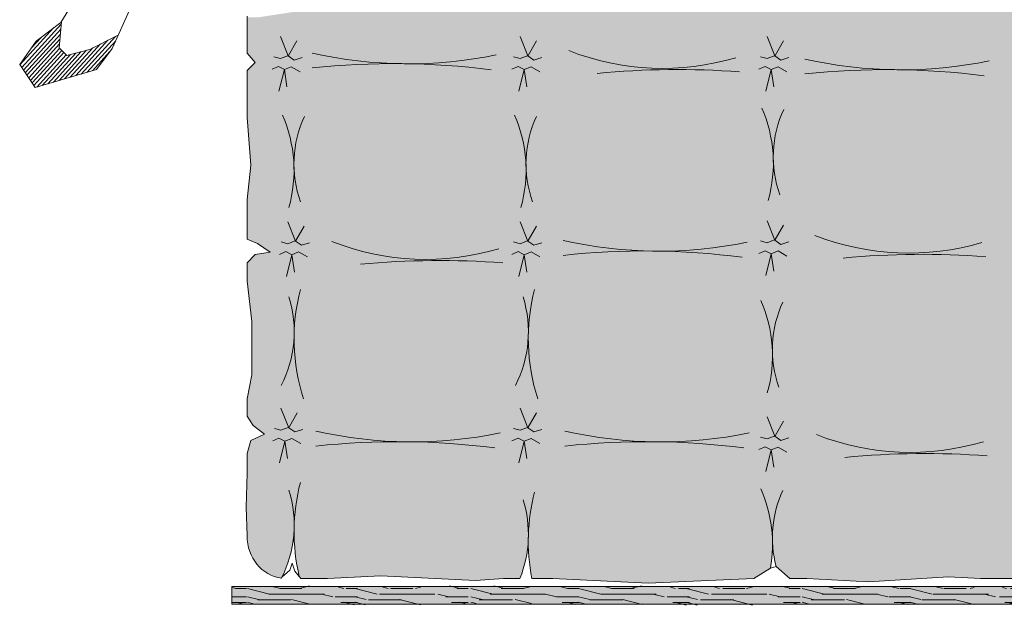
# Model space of a CAD drawing. Units: inches. Extents: x 1994 to 3075, y 3517 to 3950.
# Tile 33 of 58: x 1994.61846 to 1994.66748, y 3553.69193 to 3553.72103. Entities that reach past the tile are written whole.
import ezdxf

# ---------------------------------------------------------------- set-up
doc = ezdxf.new("R2010")
doc.units = ezdxf.units.IN
doc.layers.add('A-FURN-REFR', color=8, linetype='Continuous', lineweight=13)
doc.layers.add('A-FURN-REFR-PATT', color=8, linetype='Continuous', lineweight=13)

msp = doc.modelspace()

# ---------------------------------------------------------------- hatches: boundary and pattern name
at = {"layer": 'A-FURN-REFR-PATT'}
h = msp.add_hatch(color=256, dxfattribs=at)
h.set_gradient(color1=(238, 215, 180), color2=(243, 226, 201), one_color=1, tint=0.87)
edge = h.paths.add_edge_path()
edge.add_line((1994.681542, 3553.709525), (1994.682048, 3553.709217))
edge.add_line((1994.682048, 3553.709217), (1994.682631, 3553.708815))
edge.add_line((1994.682631, 3553.708815), (1994.682631, 3553.708383))
edge.add_line((1994.682631, 3553.708383), (1994.682498, 3553.704652))
edge.add_line((1994.682498, 3553.704652), (1994.682631, 3553.701474))
edge.add_line((1994.682631, 3553.701474), (1994.682631, 3553.700426))
edge.add_line((1994.682631, 3553.700426), (1994.682104, 3553.700396))
edge.add_line((1994.682104, 3553.700396), (1994.681598, 3553.699902))
edge.add_line((1994.681598, 3553.699902), (1994.681992, 3553.699717))
edge.add_line((1994.681992, 3553.699717), (1994.682631, 3553.699439))
edge.add_line((1994.682631, 3553.699439), (1994.682631, 3553.695334))
edge.add_ellipse((1994.680709, 3553.695334), major_axis=(0, 0.002111), ratio=0.910403, start_angle=180, end_angle=270, ccw=False)
edge.add_line((1994.680709, 3553.693223), (1994.680522, 3553.693223))
edge.add_line((1994.680522, 3553.693223), (1994.680314, 3553.694))
edge.add_ellipse((1994.68491, 3553.694998), major_axis=(0, 0.005146), ratio=0.910403, start_angle=92.3431, end_angle=102.2543, ccw=False)
edge.add_ellipse((1994.674568, 3553.694683), major_axis=(0, 0.006219), ratio=0.910403, start_angle=-88.7485, end_angle=-87.76)
edge.add_ellipse((1994.68491, 3553.694998), major_axis=(0, 0.005146), ratio=0.910403, start_angle=91.1484, end_angle=92.3431)
edge.add_ellipse((1994.674568, 3553.694683), major_axis=(0, 0.006219), ratio=0.910403, start_angle=262.8125, end_angle=271.2515, ccw=False)
edge.add_line((1994.680193, 3553.693973), (1994.679278, 3553.693223))
edge.add_line((1994.679278, 3553.693223), (1994.678042, 3553.693223))
edge.add_line((1994.678042, 3553.693223), (1994.673955, 3553.693055))
edge.add_line((1994.673955, 3553.693055), (1994.669892, 3553.693223))
edge.add_line((1994.669892, 3553.693223), (1994.669387, 3553.693223))
edge.add_line((1994.669387, 3553.693223), (1994.668536, 3553.693813))
edge.add_ellipse((1994.673095, 3553.694999), major_axis=(0, 0.005146), ratio=0.910403, start_angle=92.3431, end_angle=104.5922, ccw=False)
edge.add_ellipse((1994.662753, 3553.694684), major_axis=(0, 0.006219), ratio=0.910403, start_angle=-88.7485, end_angle=-87.76)
edge.add_ellipse((1994.673095, 3553.694999), major_axis=(0, 0.005146), ratio=0.910403, start_angle=91.1484, end_angle=92.3431)
edge.add_ellipse((1994.662753, 3553.694684), major_axis=(0, 0.006219), ratio=0.910403, start_angle=260.6759, end_angle=271.2515, ccw=False)
edge.add_line((1994.668352, 3553.693765), (1994.66822, 3553.693223))
edge.add_line((1994.66822, 3553.693223), (1994.666295, 3553.693223))
edge.add_line((1994.666295, 3553.693223), (1994.664702, 3553.693298))
edge.add_line((1994.664702, 3553.693298), (1994.660712, 3553.693051))
edge.add_line((1994.660712, 3553.693051), (1994.65764, 3553.693223))
edge.add_line((1994.65764, 3553.693223), (1994.656797, 3553.693223))
edge.add_line((1994.656797, 3553.693223), (1994.656116, 3553.693819))
edge.add_ellipse((1994.660616, 3553.695249), major_axis=(0, 0.005146), ratio=0.910403, start_angle=92.3431, end_angle=107.6246, ccw=False)
edge.add_ellipse((1994.650274, 3553.694934), major_axis=(0, 0.006219), ratio=0.910403, start_angle=-88.7485, end_angle=-87.76)
edge.add_ellipse((1994.660616, 3553.695249), major_axis=(0, 0.005146), ratio=0.910403, start_angle=91.1484, end_angle=92.3431)
edge.add_ellipse((1994.650274, 3553.694934), major_axis=(0, 0.006219), ratio=0.910403, start_angle=257.752, end_angle=271.2515, ccw=False)
edge.add_line((1994.655829, 3553.693728), (1994.654998, 3553.693223))
edge.add_line((1994.654998, 3553.693223), (1994.649752, 3553.692989))
edge.add_line((1994.649752, 3553.692989), (1994.644994, 3553.693223))
edge.add_line((1994.644994, 3553.693223), (1994.643952, 3553.693223))
edge.add_ellipse((1994.651853, 3553.695067), major_axis=(0, 0.008872), ratio=0.910403, start_angle=89.8354, end_angle=103.1369, ccw=False)
edge.add_ellipse((1994.638929, 3553.695405), major_axis=(0, 0.005332), ratio=0.910403, start_angle=266.2788, end_angle=270.7223)
edge.add_ellipse((1994.651853, 3553.695067), major_axis=(0, 0.008872), ratio=0.910403, start_angle=87.1651, end_angle=89.8354)
edge.add_ellipse((1994.638929, 3553.695405), major_axis=(0, 0.005332), ratio=0.910403, start_angle=243.7698, end_angle=266.2788, ccw=False)
edge.add_line((1994.643359, 3553.693223), (1994.642545, 3553.693223))
edge.add_line((1994.642545, 3553.693223), (1994.641153, 3553.693113))
edge.add_line((1994.641153, 3553.693113), (1994.636432, 3553.693359))
edge.add_line((1994.636432, 3553.693359), (1994.633777, 3553.693223))
edge.add_line((1994.633777, 3553.693223), (1994.63245, 3553.693223))
edge.add_line((1994.63245, 3553.693223), (1994.632375, 3553.693314))
edge.add_ellipse((1994.640193, 3553.695548), major_axis=(0, 0.008872), ratio=0.910403, start_angle=89.8354, end_angle=105.9456, ccw=False)
edge.add_ellipse((1994.627269, 3553.695886), major_axis=(0, 0.005332), ratio=0.910403, start_angle=266.2788, end_angle=270.7223)
edge.add_ellipse((1994.640193, 3553.695548), major_axis=(0, 0.008872), ratio=0.910403, start_angle=87.1651, end_angle=89.8354)
edge.add_ellipse((1994.627269, 3553.695886), major_axis=(0, 0.005332), ratio=0.910403, start_angle=237.8324, end_angle=266.2788, ccw=False)
edge.add_ellipse((1994.6317, 3553.695334), major_axis=(0, 0.002111), ratio=0.910403, start_angle=90, end_angle=174.0631, ccw=False)
edge.add_line((1994.629778, 3553.695334), (1994.629737, 3553.696763))
edge.add_line((1994.629737, 3553.696763), (1994.629778, 3553.698454))
edge.add_line((1994.629778, 3553.698454), (1994.629778, 3553.699441))
edge.add_line((1994.629778, 3553.699441), (1994.629962, 3553.700094))
edge.add_line((1994.629962, 3553.700094), (1994.630637, 3553.700403))
edge.add_line((1994.630637, 3553.700403), (1994.630075, 3553.700834))
edge.add_line((1994.630075, 3553.700834), (1994.629778, 3553.701292))
edge.add_line((1994.629778, 3553.701292), (1994.629778, 3553.702155))
edge.add_line((1994.629778, 3553.702155), (1994.630018, 3553.703363))
edge.add_line((1994.630018, 3553.703363), (1994.630018, 3553.706016))
edge.add_line((1994.630018, 3553.706016), (1994.629778, 3553.708015))
edge.add_line((1994.629778, 3553.708015), (1994.629778, 3553.70894))
edge.add_line((1994.629778, 3553.70894), (1994.630187, 3553.709347))
edge.add_line((1994.630187, 3553.709347), (1994.630918, 3553.70947))
edge.add_line((1994.630918, 3553.70947), (1994.630299, 3553.709902))
edge.add_line((1994.630299, 3553.709902), (1994.629778, 3553.710112))
edge.add_line((1994.629778, 3553.710112), (1994.629778, 3553.712086))
edge.add_line((1994.629778, 3553.712086), (1994.629962, 3553.713788))
edge.add_line((1994.629962, 3553.713788), (1994.629778, 3553.716158))
edge.add_line((1994.629778, 3553.716158), (1994.629778, 3553.718502))
edge.add_line((1994.629778, 3553.718502), (1994.630187, 3553.718908))
edge.add_line((1994.630187, 3553.718908), (1994.629778, 3553.719365))
edge.add_line((1994.629778, 3553.719365), (1994.629778, 3553.72115))
edge.add_line((1994.629778, 3553.72115), (1994.630322, 3553.72115))
edge.add_line((1994.630322, 3553.72115), (1994.634865, 3553.721849))
edge.add_line((1994.634865, 3553.721849), (1994.639494, 3553.724204))
edge.add_line((1994.639494, 3553.724204), (1994.643653, 3553.725608))
edge.add_ellipse((1994.63891, 3553.72447), major_axis=(0, 0.005332), ratio=0.910403, start_angle=270.7223, end_angle=283.4893, ccw=False)
edge.add_ellipse((1994.651833, 3553.724132), major_axis=(0, 0.008872), ratio=0.910403, start_angle=87.1651, end_angle=89.8354)
edge.add_ellipse((1994.63891, 3553.72447), major_axis=(0, 0.005332), ratio=0.910403, start_angle=266.2788, end_angle=270.7223)
edge.add_ellipse((1994.651833, 3553.724132), major_axis=(0, 0.008872), ratio=0.910403, start_angle=438.9501, end_angle=447.1651, ccw=False)
edge.add_line((1994.643881, 3553.725685), (1994.643897, 3553.72569))
edge.add_line((1994.643897, 3553.72569), (1994.649542, 3553.726806))
edge.add_line((1994.649542, 3553.726806), (1994.655977, 3553.727797))
edge.add_line((1994.655977, 3553.727797), (1994.658348, 3553.728382))
edge.add_ellipse((1994.662052, 3553.754177), major_axis=(0, 0.026115), ratio=0.910403, start_angle=171.8281, end_angle=180.2609)
edge.add_ellipse((1994.661314, 3553.682223), major_axis=(0, 0.04585), ratio=0.910403, start_angle=-1.0711, end_angle=-0.1044)
edge.add_ellipse((1994.662052, 3553.754177), major_axis=(0, 0.026115), ratio=0.910403, start_angle=171.8281, end_angle=178.5636, ccw=False)
edge.add_line((1994.658348, 3553.728382), (1994.666025, 3553.730275))
edge.add_line((1994.666025, 3553.730275), (1994.67483, 3553.732877))
edge.add_line((1994.67483, 3553.732877), (1994.680219, 3553.734687))
edge.add_ellipse((1994.675489, 3553.733489), major_axis=(0, 0.005332), ratio=0.910403, start_angle=270.7223, end_angle=284.2178, ccw=False)
edge.add_ellipse((1994.688412, 3553.73315), major_axis=(0, 0.008872), ratio=0.910403, start_angle=87.1651, end_angle=89.8354)
edge.add_ellipse((1994.675489, 3553.733489), major_axis=(0, 0.005332), ratio=0.910403, start_angle=266.2788, end_angle=270.7223)
edge.add_ellipse((1994.688412, 3553.73315), major_axis=(0, 0.008872), ratio=0.910403, start_angle=438.5005, end_angle=447.1651, ccw=False)
edge.add_line((1994.68047, 3553.734766), (1994.682205, 3553.735263))
edge.add_line((1994.682205, 3553.735263), (1994.682631, 3553.735263))
edge.add_line((1994.682631, 3553.735263), (1994.682631, 3553.734609))
edge.add_line((1994.682631, 3553.734609), (1994.682783, 3553.733623))
edge.add_line((1994.682783, 3553.733623), (1994.682631, 3553.730537))
edge.add_line((1994.682631, 3553.730537), (1994.682631, 3553.728749))
edge.add_line((1994.682631, 3553.728749), (1994.682334, 3553.728195))
edge.add_line((1994.682334, 3553.728195), (1994.681547, 3553.727824))
edge.add_line((1994.681547, 3553.727824), (1994.682053, 3553.727639))
edge.add_line((1994.682053, 3553.727639), (1994.682631, 3553.72733))
edge.add_line((1994.682631, 3553.72733), (1994.682631, 3553.725726))
edge.add_line((1994.682631, 3553.725726), (1994.682727, 3553.724308))
edge.add_line((1994.682727, 3553.724308), (1994.682631, 3553.721716))
edge.add_line((1994.682631, 3553.721716), (1994.682631, 3553.720165))
edge.add_line((1994.682631, 3553.720165), (1994.682329, 3553.719086))
edge.add_line((1994.682329, 3553.719086), (1994.681823, 3553.718654))
edge.add_line((1994.681823, 3553.718654), (1994.682329, 3553.718531))
edge.add_line((1994.682329, 3553.718531), (1994.682722, 3553.718346))
edge.add_line((1994.682722, 3553.718346), (1994.68261, 3553.715693))
edge.add_line((1994.68261, 3553.715693), (1994.682631, 3553.711159))
edge.add_line((1994.682631, 3553.711159), (1994.682631, 3553.710327))
edge.add_line((1994.682631, 3553.710327), (1994.682217, 3553.70971))
edge.add_line((1994.682217, 3553.70971), (1994.681542, 3553.709525))
edge = h.paths.add_edge_path(flags=16)
edge.add_ellipse((1994.674017, 3553.663488), major_axis=(0, 0.04585), ratio=0.910403, start_angle=-1.0711, end_angle=-0.1044)
edge.add_ellipse((1994.674755, 3553.735442), major_axis=(0, 0.026115), ratio=0.910403, start_angle=178.5636, end_angle=180.2609)
h.paths.add_polyline_path([(1994.668419, 3553.710039), (1994.668385, 3553.710026), (1994.668404, 3553.710013)], flags=16)
edge = h.paths.add_edge_path(flags=16)
edge.add_ellipse((1994.663397, 3553.714852), major_axis=(0, 0.005332), ratio=0.910403, start_angle=266.2788, end_angle=270.7223)
edge.add_ellipse((1994.67632, 3553.714514), major_axis=(0, 0.008872), ratio=0.910403, start_angle=87.1651, end_angle=89.8354)
edge = h.paths.add_edge_path(flags=16)
edge.add_ellipse((1994.662753, 3553.703926), major_axis=(0, 0.006219), ratio=0.910403, start_angle=-88.7485, end_angle=-87.76)
edge.add_ellipse((1994.673095, 3553.704241), major_axis=(0, 0.005146), ratio=0.910403, start_angle=91.1484, end_angle=92.3431)
h.paths.add_polyline_path([(1994.680357, 3553.710026), (1994.680376, 3553.710013), (1994.680391, 3553.710039)], flags=16)
edge = h.paths.add_edge_path(flags=16)
edge.add_ellipse((1994.684791, 3553.713857), major_axis=(0, 0.005146), ratio=0.910403, start_angle=91.1484, end_angle=92.3431)
edge.add_ellipse((1994.67445, 3553.713542), major_axis=(0, 0.006219), ratio=0.910403, start_angle=-88.7485, end_angle=-87.76)
h.paths.add_polyline_path([(1994.668404, 3553.719229), (1994.668419, 3553.719256), (1994.668385, 3553.719242)], flags=16)
edge = h.paths.add_edge_path(flags=16)
edge.add_ellipse((1994.68491, 3553.704625), major_axis=(0, 0.005146), ratio=0.910403, start_angle=91.1484, end_angle=92.3431)
edge.add_ellipse((1994.674568, 3553.70431), major_axis=(0, 0.006219), ratio=0.910403, start_angle=-88.7485, end_angle=-87.76)
edge = h.paths.add_edge_path(flags=16)
edge.add_ellipse((1994.662353, 3553.744655), major_axis=(0, 0.026115), ratio=0.910403, start_angle=178.5636, end_angle=180.2609)
edge.add_ellipse((1994.661615, 3553.6727), major_axis=(0, 0.04585), ratio=0.910403, start_angle=-1.0711, end_angle=-0.1044)
edge = h.paths.add_edge_path(flags=16)
edge.add_ellipse((1994.662621, 3553.722979), major_axis=(0, 0.006219), ratio=0.910403, start_angle=-88.7485, end_angle=-87.76)
edge.add_ellipse((1994.672963, 3553.723294), major_axis=(0, 0.005146), ratio=0.910403, start_angle=91.1484, end_angle=92.3431)
h.paths.add_polyline_path([(1994.68017, 3553.719242), (1994.680189, 3553.719229), (1994.680204, 3553.719256)], flags=16)
h.paths.add_polyline_path([(1994.668419, 3553.70036), (1994.668385, 3553.700347), (1994.668404, 3553.700334)], flags=16)
edge = h.paths.add_edge_path(flags=16)
edge.add_ellipse((1994.673942, 3553.654177), major_axis=(0, 0.04585), ratio=0.910403, start_angle=-1.0711, end_angle=-0.1044)
edge.add_ellipse((1994.67468, 3553.726132), major_axis=(0, 0.026115), ratio=0.910403, start_angle=178.5636, end_angle=180.2609)
edge = h.paths.add_edge_path(flags=16)
edge.add_ellipse((1994.685026, 3553.723294), major_axis=(0, 0.005146), ratio=0.910403, start_angle=91.1484, end_angle=92.3431)
edge.add_ellipse((1994.674684, 3553.722979), major_axis=(0, 0.006219), ratio=0.910403, start_angle=-88.7485, end_angle=-87.76)
h.paths.add_polyline_path([(1994.680569, 3553.70036), (1994.680535, 3553.700347), (1994.680554, 3553.700334)], flags=16)
h.paths.add_polyline_path([(1994.656068, 3553.710085), (1994.656034, 3553.710071), (1994.656052, 3553.710058)], flags=16)
h.paths.add_polyline_path([(1994.668404, 3553.728426), (1994.668419, 3553.728453), (1994.668385, 3553.728439)], flags=16)
edge = h.paths.add_edge_path(flags=16)
edge.add_ellipse((1994.650317, 3553.713896), major_axis=(0, 0.006219), ratio=0.910403, start_angle=-88.7485, end_angle=-87.76)
edge.add_ellipse((1994.660659, 3553.714211), major_axis=(0, 0.005146), ratio=0.910403, start_angle=91.1484, end_angle=92.3431)
edge = h.paths.add_edge_path(flags=16)
edge.add_ellipse((1994.650274, 3553.70431), major_axis=(0, 0.006219), ratio=0.910403, start_angle=-88.7485, end_angle=-87.76)
edge.add_ellipse((1994.660616, 3553.704625), major_axis=(0, 0.005146), ratio=0.910403, start_angle=91.1484, end_angle=92.3431)
h.paths.add_polyline_path([(1994.68033, 3553.728439), (1994.680349, 3553.728426), (1994.680364, 3553.728453)], flags=16)
h.paths.add_polyline_path([(1994.656052, 3553.719229), (1994.656068, 3553.719256), (1994.656034, 3553.719242)], flags=16)
edge = h.paths.add_edge_path(flags=16)
edge.add_ellipse((1994.649569, 3553.663672), major_axis=(0, 0.04585), ratio=0.910403, start_angle=-1.0711, end_angle=-0.1044)
edge.add_ellipse((1994.650307, 3553.735627), major_axis=(0, 0.026115), ratio=0.910403, start_angle=178.5636, end_angle=180.2609)
h.paths.add_polyline_path([(1994.656068, 3553.700324), (1994.656034, 3553.70031), (1994.656052, 3553.700297)], flags=16)
edge = h.paths.add_edge_path(flags=16)
edge.add_ellipse((1994.650446, 3553.723545), major_axis=(0, 0.006219), ratio=0.910403, start_angle=-88.7485, end_angle=-87.76)
edge.add_ellipse((1994.660788, 3553.72386), major_axis=(0, 0.005146), ratio=0.910403, start_angle=91.1484, end_angle=92.3431)
edge = h.paths.add_edge_path(flags=16)
edge.add_ellipse((1994.64966, 3553.654177), major_axis=(0, 0.04585), ratio=0.910403, start_angle=-1.0711, end_angle=-0.1044)
edge.add_ellipse((1994.650398, 3553.726132), major_axis=(0, 0.026115), ratio=0.910403, start_angle=178.5636, end_angle=180.2609)
h.paths.add_polyline_path([(1994.643774, 3553.710039), (1994.64374, 3553.710026), (1994.643759, 3553.710013)], flags=16)
edge = h.paths.add_edge_path(flags=16)
edge.add_ellipse((1994.638006, 3553.713542), major_axis=(0, 0.006219), ratio=0.910403, start_angle=-88.7485, end_angle=-87.76)
edge.add_ellipse((1994.648347, 3553.713857), major_axis=(0, 0.005146), ratio=0.910403, start_angle=91.1484, end_angle=92.3431)
edge = h.paths.add_edge_path(flags=16)
edge.add_ellipse((1994.638929, 3553.705498), major_axis=(0, 0.005332), ratio=0.910403, start_angle=266.2788, end_angle=270.7223)
edge.add_ellipse((1994.651853, 3553.705159), major_axis=(0, 0.008872), ratio=0.910403, start_angle=87.1651, end_angle=89.8354)
h.paths.add_polyline_path([(1994.643759, 3553.719229), (1994.643774, 3553.719256), (1994.64374, 3553.719242)], flags=16)
h.paths.add_polyline_path([(1994.643774, 3553.700752), (1994.64374, 3553.700739), (1994.643759, 3553.700726)], flags=16)
edge = h.paths.add_edge_path(flags=16)
edge.add_ellipse((1994.637078, 3553.672998), major_axis=(0, 0.04585), ratio=0.910403, start_angle=-1.0711, end_angle=-0.1044)
edge.add_ellipse((1994.637816, 3553.744953), major_axis=(0, 0.026115), ratio=0.910403, start_angle=178.5636, end_angle=180.2609)
edge = h.paths.add_edge_path(flags=16)
edge.add_ellipse((1994.637265, 3553.654177), major_axis=(0, 0.04585), ratio=0.910403, start_angle=-1.0711, end_angle=-0.1044)
edge.add_ellipse((1994.638003, 3553.726132), major_axis=(0, 0.026115), ratio=0.910403, start_angle=178.5636, end_angle=180.2609)
h.paths.add_polyline_path([(1994.632201, 3553.710039), (1994.632167, 3553.710026), (1994.632186, 3553.710013)], flags=16)
edge = h.paths.add_edge_path(flags=16)
edge.add_ellipse((1994.626452, 3553.713542), major_axis=(0, 0.006219), ratio=0.910403, start_angle=-88.7485, end_angle=-87.76)
edge.add_ellipse((1994.636794, 3553.713857), major_axis=(0, 0.005146), ratio=0.910403, start_angle=91.1484, end_angle=92.3431)
edge = h.paths.add_edge_path(flags=16)
edge.add_ellipse((1994.627269, 3553.705498), major_axis=(0, 0.005332), ratio=0.910403, start_angle=266.2788, end_angle=270.7223)
edge.add_ellipse((1994.640193, 3553.705159), major_axis=(0, 0.008872), ratio=0.910403, start_angle=87.1651, end_angle=89.8354)
h.paths.add_polyline_path([(1994.631818, 3553.719229), (1994.631834, 3553.719256), (1994.631799, 3553.719242)], flags=16)
h.paths.add_polyline_path([(1994.631864, 3553.700752), (1994.63183, 3553.700739), (1994.631849, 3553.700726)], flags=16)
h = msp.add_hatch(dxfattribs=at)
h.set_pattern_fill('ANSI31', color=256, scale=0.001151, angle=-0.07, style=0)
h.set_pattern_definition([(47.6851648, (1992.79633966, 3550.73205381), (0.000101908402, -0.0001119376326), [])])
h.paths.add_polyline_path([(1994.619276, 3553.71997), (1994.620529, 3553.720911), (1994.620427, 3553.719626), (1994.620805, 3553.719254), (1994.621939, 3553.719557), (1994.623362, 3553.720268), (1994.623066, 3553.719605), (1994.622277, 3553.71855), (1994.61923, 3553.717661), (1994.618455, 3553.7188)])
msp.add_hatch(color=256, dxfattribs=at).paths.add_polyline_path([(1994.683555, 3553.692818), (1994.629017, 3553.692818), (1994.629017, 3553.691934), (1994.683555, 3553.691934)])
h = msp.add_hatch(dxfattribs=at)
h.set_pattern_fill('LEGNO1', color=256, scale=0.005512, style=0, pattern_type=2)
h.set_pattern_definition([(0, (2000.7131367, 3549.9540566), (0, 0.005511811), [0.0011023622, -0.0016535433, 0.000551181, -0.0022047244]), (0, (2000.716995, 3549.9541944), (0, 0.005511811), [0.001102362, -0.004409449]), (0, (2000.716444, 3549.95447), (0, 0.005511811), [0.000551181, -0.00496063]), (0, (2000.713412, 3549.954608), (0, 0.005511811), [0.0002755906, -0.0038582677, 0.0002755906, -0.0011023622]), (0, (2000.7153414, 3549.9548834), (0, 0.005511811), [0.0011023622, -0.0016535433, 0.0002755906, -0.002480315]), (0, (2000.7139634, 3549.955021), (0, 0.005511811), [0.0008267717, -0.0046850394]), (0, (2000.7153414, 3549.955159), (0, 0.005511811), [0.0016535433, -0.0038582677]), (0, (2000.713688, 3549.955297), (0, 0.005511811), [0.001102362, -0.004409449]), (0, (2000.7158926, 3549.9554346), (0, 0.005511811), [0.0027559055, -0.0027559055]), (0, (2000.714239, 3549.95571), (0, 0.005511811), [0.000551181, -0.0016535433, 0.0011023622, -0.0022047244]), (0, (2000.7180973, 3549.955848), (0, 0.005511811), [0.001102362, -0.004409449]), (0, (2000.716995, 3549.955986), (0, 0.005511811), [0.000551181, -0.00496063]), (0, (2000.7158926, 3549.9561236), (0, 0.005511811), [0.000551181, -0.00496063]), (0, (2000.7131367, 3549.9562614), (0, 0.005511811), [0.001102362, -0.004409449]), (0, (2000.7158926, 3549.956399), (0, 0.005511811), [0.001102362, -0.004409449]), (0, (2000.7158926, 3549.956675), (0, 0.005511811), [0.0011023622, -0.0011023622, 0.0011023622, -0.0022047244]), (0, (2000.71479, 3549.9569503), (0, 0.005511811), [0.000551181, -0.0027559055, 0.0011023622, -0.0011023622]), (0, (2000.7158926, 3549.957088), (0, 0.005511811), [0.0016535433, -0.0038582677]), (0, (2000.7158926, 3549.957364), (0, 0.005511811), [0.001102362, -0.004409449]), (0, (2000.713688, 3549.9575015), (0, 0.005511811), [0.0016535433, -0.0022047244, 0.000551181, -0.0011023622]), (0, (2000.713688, 3549.957777), (0, 0.005511811), [0.0027559055, -0.0027559055]), (0, (2000.716995, 3549.957915), (0, 0.005511811), [0.000551181, -0.00496063]), (0, (2000.7153414, 3549.9580527), (0, 0.005511811), [0.001102362, -0.004409449]), (0, (2000.714239, 3549.9581905), (0, 0.005511811), [0.000551181, -0.0022047244, 0.000551181, -0.0022047244]), (0, (2000.713688, 3549.9583283), (0, 0.005511811), [0.000551181, -0.0016535433, 0.0011023622, -0.0022047244]), (0, (2000.71479, 3549.958466), (0, 0.005511811), [0.000551181, -0.0027559055, 0.000551181, -0.0016535433]), (0, (2000.7158926, 3549.958604), (0, 0.005511811), [0.0016535433, -0.0038582677]), (0, (2000.713688, 3549.9588795), (0, 0.005511811), [0.001102362, -0.004409449]), (0, (2000.716444, 3549.959017), (0, 0.005511811), [0.000551181, -0.00496063]), (0, (2000.717546, 3549.959155), (0, 0.005511811), [0.000551181, -0.00496063]), (14.036243, (2000.7169949, 3549.95447), (0.00551181102, -2e-13), [0.0005677165, -0.022158062]), (14.036243, (2000.7175461, 3549.9557102), (0.00551181102, -2e-13), [0.0005677165, -0.022158062]), (14.036243, (2000.7169949, 3549.9590173), (0.00551181102, -2e-13), [0.0005677165, -0.022158062]), (14.036243, (2000.7153414, 3549.9569503), (0.00551181102, -2e-13), [0.0005677165, -0.022158062]), (14.036243, (2000.7164437, 3549.9577771), (0.00551181102, -2e-13), [0.0005677165, -0.022158062]), (14.036243, (2000.7169949, 3549.9573637), (0.00551181102, -2e-13), [0.0005677165, -0.022158062]), (14.036243, (2000.714239, 3549.9583283), (0.00551181102, -2e-13), [0.0005677165, -0.022158062]), (14.036243, (2000.7164437, 3549.9580527), (0.00551181102, -2e-13), [0.0005677165, -0.022158062]), (14.036243, (2000.7175461, 3549.9559858), (0.00551181102, -2e-13), [0.001135433, -0.0215903454]), (14.036243, (2000.7169949, 3549.9563992), (0.00551181102, -2e-13), [0.001135433, -0.0215903454]), (14.036243, (2000.7169949, 3549.9566748), (0.00551181102, -2e-13), [0.001135433, -0.0215903454]), (165.963757, (2000.7153414, 3549.9548834), (-0.00551181102, -2e-13), [0.0005677165, -0.001135433, 0.0005677165, -0.0204549123]), (165.963757, (2000.714239, 3549.9557102), (-0.00551181102, -2e-13), [0.0005677165, -0.022158062]), (165.963757, (2000.714239, 3549.9581905), (-0.00551181102, -2e-13), [0.001135433, -0.0215903454]), (194.036243, (2000.7169949, 3549.9541944), (-0.00551181102, 2e-13), [0.0005677165, -0.022158062]), (345.963757, (2000.7180973, 3549.9541944), (0.00551181102, 2e-13), [0.0005677165, -0.022158062]), (345.963757, (2000.7164437, 3549.9561236), (0.00551181102, 2e-13), [0.0005677165, -0.022158062]), (345.963757, (2000.7175461, 3549.9570881), (0.00551181102, 2e-13), [0.0005677165, -0.022158062]), (345.963757, (2000.7153414, 3549.9575015), (0.00551181102, 2e-13), [0.0005677165, -0.022158062]), (345.963757, (2000.7147902, 3549.9581905), (0.00551181102, 2e-13), [0.0005677165, -0.022158062]), (345.963757, (2000.7153414, 3549.9584661), (0.00551181102, 2e-13), [0.0005677165, -0.022158062]), (345.963757, (2000.7153414, 3549.9575015), (0.00551181102, 2e-13), [0.0005677165, -0.022158062]), (345.963757, (2000.7169949, 3549.9583283), (0.00551181102, 2e-13), [0.002270866, -0.0204549123]), (345.963757, (2000.7136878, 3549.9546078), (0.00551181102, 2e-13), [0.002270866, -0.0204549123]), (345.963757, (2000.714239, 3549.9550212), (0.00551181102, 2e-13), [0.002270866, -0.0204549123]), (345.963757, (2000.7147902, 3549.9552968), (0.00551181102, 2e-13), [0.0005677165, -0.001135433, 0.001135433, -0.0198871958]), (345.963757, (2000.7147902, 3549.9557102), (0.00551181102, 2e-13), [0.001135433, -0.001135433, 0.001135433, -0.0193194793]), (345.963757, (2000.714239, 3549.9562614), (0.00551181102, 2e-13), [0.002270866, -0.0204549123]), (345.963757, (2000.7136878, 3549.9566748), (0.00551181102, 2e-13), [0.002270866, -0.0204549123]), (345.963757, (2000.7136878, 3549.9569503), (0.00551181102, 2e-13), [0.002270866, -0.0204549123]), (345.963757, (2000.7175461, 3549.9586039), (0.00551181102, 2e-13), [0.0005677165, -0.022158062]), (345.963768, (2000.7180973, 3549.959155), (0.00551181102, 1.06e-09), [0.001135433, -0.0215903454]), (345.963768, (2000.7147902, 3549.9588795), (0.00551181102, 1.06e-09), [0.001135433, -0.0215903454]), (345.963758, (2000.714239, 3549.9540566), (0.00551181102, 1e-10), [0.002270866, -0.0204549123]), (345.963758, (2000.7175461, 3549.9579149), (0.00551181102, 1e-10), [0.0017031496, -0.021022629]), (345.963758, (2000.7180973, 3549.9575015), (0.00551181102, 1e-10), [0.0034062992, -0.0193194793])])
h.paths.add_polyline_path([(1994.683555, 3553.692818), (1994.629017, 3553.692818), (1994.629017, 3553.691934), (1994.683555, 3553.691934)])

# ---------------------------------------------------------------- linework, layer by layer
at = {"layer": 'A-FURN-REFR'}
for p, q in [((1994.620508, 3553.720895), (1994.621306, 3553.722205)), ((1994.623992, 3553.721652), (1994.623473, 3553.720516)), ((1994.629778, 3553.719365), (1994.629778, 3553.721215)), ((1994.619276, 3553.71997), (1994.620508, 3553.720895)), ((1994.620531, 3553.720932), (1994.620427, 3553.719626)), ((1994.621939, 3553.719557), (1994.623362, 3553.720268)), ((1994.623473, 3553.720516), (1994.623066, 3553.719605)), ((1994.631818, 3553.719229), (1994.631434, 3553.720195)), ((1994.643759, 3553.719229), (1994.643375, 3553.720195)), ((1994.656052, 3553.719229), (1994.655669, 3553.720195)), ((1994.618455, 3553.7188), (1994.619276, 3553.71997)), ((1994.631834, 3553.719256), (1994.632247, 3553.719976)), ((1994.643774, 3553.719256), (1994.644187, 3553.719976)), ((1994.656068, 3553.719256), (1994.656481, 3553.719976)), ((1994.620427, 3553.719626), (1994.620805, 3553.719254)), ((1994.620805, 3553.719254), (1994.621939, 3553.719557)), ((1994.623066, 3553.719605), (1994.622277, 3553.71855)), ((1994.629778, 3553.719365), (1994.630187, 3553.718908)), ((1994.631107, 3553.719193), (1994.631434, 3553.719099)), ((1994.631434, 3553.719099), (1994.631834, 3553.719256)), ((1994.632119, 3553.719021), (1994.631818, 3553.719229)), ((1994.643047, 3553.719193), (1994.643375, 3553.719099)), ((1994.643375, 3553.719099), (1994.643774, 3553.719256)), ((1994.644059, 3553.719021), (1994.643759, 3553.719229)), ((1994.655341, 3553.719193), (1994.655669, 3553.719099)), ((1994.655669, 3553.719099), (1994.656068, 3553.719256)), ((1994.656353, 3553.719021), (1994.656052, 3553.719229)), ((1994.61923, 3553.717661), (1994.618455, 3553.7188)), ((1994.630187, 3553.718908), (1994.629778, 3553.718502)), ((1994.631021, 3553.718567), (1994.631335, 3553.718708)), ((1994.631335, 3553.718708), (1994.631634, 3553.718552)), ((1994.631976, 3553.718693), (1994.631634, 3553.718552)), ((1994.632418, 3553.718442), (1994.631976, 3553.718693)), ((1994.632518, 3553.719146), (1994.632119, 3553.719021)), ((1994.642961, 3553.718567), (1994.643275, 3553.718708)), ((1994.643275, 3553.718708), (1994.643574, 3553.718552)), ((1994.643916, 3553.718693), (1994.643574, 3553.718552)), ((1994.644358, 3553.718442), (1994.643916, 3553.718693)), ((1994.644458, 3553.719146), (1994.644059, 3553.719021)), ((1994.655255, 3553.718567), (1994.655569, 3553.718708)), ((1994.655569, 3553.718708), (1994.655868, 3553.718552)), ((1994.65621, 3553.718693), (1994.655868, 3553.718552)), ((1994.656652, 3553.718442), (1994.65621, 3553.718693)), ((1994.656752, 3553.719146), (1994.656353, 3553.719021)), ((1994.622277, 3553.71855), (1994.61923, 3553.717661)), ((1994.629778, 3553.716158), (1994.629778, 3553.718502)), ((1994.631634, 3553.718552), (1994.631363, 3553.717472)), ((1994.631634, 3553.718552), (1994.631762, 3553.717691)), ((1994.643574, 3553.718552), (1994.643303, 3553.717472)), ((1994.643574, 3553.718552), (1994.643702, 3553.717691)), ((1994.655868, 3553.718552), (1994.655597, 3553.717472)), ((1994.655868, 3553.718552), (1994.655996, 3553.717691)), ((1994.629778, 3553.716158), (1994.629962, 3553.713788)), ((1994.629962, 3553.713788), (1994.629778, 3553.712086)), ((1994.629778, 3553.710112), (1994.629778, 3553.712086)), ((1994.632186, 3553.710013), (1994.631802, 3553.710978)), ((1994.643759, 3553.710013), (1994.643375, 3553.710978)), ((1994.656052, 3553.710058), (1994.655669, 3553.711023)), ((1994.632201, 3553.710039), (1994.632614, 3553.710759)), ((1994.643774, 3553.710039), (1994.644187, 3553.710759)), ((1994.656068, 3553.710085), (1994.656481, 3553.710804)), ((1994.629778, 3553.710112), (1994.630299, 3553.709902)), ((1994.630299, 3553.709902), (1994.630918, 3553.70947)), ((1994.631474, 3553.709977), (1994.631802, 3553.709883)), ((1994.631802, 3553.709883), (1994.632201, 3553.710039)), ((1994.632486, 3553.709804), (1994.632186, 3553.710013)), ((1994.632885, 3553.70993), (1994.632486, 3553.709804)), ((1994.643047, 3553.709977), (1994.643375, 3553.709883)), ((1994.643375, 3553.709883), (1994.643774, 3553.710039)), ((1994.644059, 3553.709804), (1994.643759, 3553.710013)), ((1994.644458, 3553.70993), (1994.644059, 3553.709804)), ((1994.655341, 3553.710022), (1994.655669, 3553.709928)), ((1994.655669, 3553.709928), (1994.656068, 3553.710085)), ((1994.656353, 3553.70985), (1994.656052, 3553.710058)), ((1994.656752, 3553.709975), (1994.656353, 3553.70985)), ((1994.630918, 3553.70947), (1994.630187, 3553.709347)), ((1994.631388, 3553.709351), (1994.631702, 3553.709492)), ((1994.631702, 3553.709492), (1994.632001, 3553.709335)), ((1994.632344, 3553.709476), (1994.632001, 3553.709335)), ((1994.632786, 3553.709226), (1994.632344, 3553.709476)), ((1994.642961, 3553.709351), (1994.643275, 3553.709492)), ((1994.643275, 3553.709492), (1994.643574, 3553.709335)), ((1994.643916, 3553.709476), (1994.643574, 3553.709335)), ((1994.644358, 3553.709226), (1994.643916, 3553.709476)), ((1994.655255, 3553.709396), (1994.655569, 3553.709537)), ((1994.655569, 3553.709537), (1994.655868, 3553.709381)), ((1994.655868, 3553.709381), (1994.655597, 3553.708301)), ((1994.65621, 3553.709521), (1994.655868, 3553.709381)), ((1994.655868, 3553.709381), (1994.655996, 3553.70852)), ((1994.656652, 3553.709271), (1994.65621, 3553.709521)), ((1994.630187, 3553.709347), (1994.629778, 3553.70894)), ((1994.629778, 3553.708015), (1994.629778, 3553.70894)), ((1994.632001, 3553.709335), (1994.631731, 3553.708255)), ((1994.632001, 3553.709335), (1994.63213, 3553.708474)), ((1994.643574, 3553.709335), (1994.643303, 3553.708255)), ((1994.643574, 3553.709335), (1994.643702, 3553.708474)), ((1994.629778, 3553.708015), (1994.630018, 3553.706016)), ((1994.630018, 3553.706016), (1994.630018, 3553.703363)), ((1994.630018, 3553.703363), (1994.629778, 3553.702155)), ((1994.629778, 3553.701292), (1994.629778, 3553.702155)), ((1994.631849, 3553.700726), (1994.631465, 3553.701691)), ((1994.643759, 3553.700726), (1994.643375, 3553.701691)), ((1994.629778, 3553.701292), (1994.630075, 3553.700834)), ((1994.631864, 3553.700752), (1994.632277, 3553.701472)), ((1994.643774, 3553.700752), (1994.644187, 3553.701472)), ((1994.656052, 3553.700297), (1994.655669, 3553.701262)), ((1994.656068, 3553.700324), (1994.656481, 3553.701043)), ((1994.630075, 3553.700834), (1994.630637, 3553.700403)), ((1994.631137, 3553.700689), (1994.631465, 3553.700596)), ((1994.631465, 3553.700596), (1994.631864, 3553.700752)), ((1994.632149, 3553.700517), (1994.631849, 3553.700726)), ((1994.632548, 3553.700643), (1994.632149, 3553.700517)), ((1994.643047, 3553.700689), (1994.643375, 3553.700596)), ((1994.643375, 3553.700596), (1994.643774, 3553.700752)), ((1994.644059, 3553.700517), (1994.643759, 3553.700726)), ((1994.644458, 3553.700643), (1994.644059, 3553.700517)), ((1994.629962, 3553.700094), (1994.629778, 3553.699441)), ((1994.630637, 3553.700403), (1994.629962, 3553.700094)), ((1994.631051, 3553.700064), (1994.631365, 3553.700204)), ((1994.631365, 3553.700204), (1994.631664, 3553.700048)), ((1994.631664, 3553.700048), (1994.631393, 3553.698968)), ((1994.632006, 3553.700189), (1994.631664, 3553.700048)), ((1994.631664, 3553.700048), (1994.631792, 3553.699187)), ((1994.632448, 3553.699938), (1994.632006, 3553.700189)), ((1994.642961, 3553.700064), (1994.643275, 3553.700204)), ((1994.643275, 3553.700204), (1994.643574, 3553.700048)), ((1994.643574, 3553.700048), (1994.643303, 3553.698968)), ((1994.643916, 3553.700189), (1994.643574, 3553.700048)), ((1994.643574, 3553.700048), (1994.643702, 3553.699187)), ((1994.644358, 3553.699938), (1994.643916, 3553.700189)), ((1994.655341, 3553.700261), (1994.655669, 3553.700167)), ((1994.655669, 3553.700167), (1994.656068, 3553.700324)), ((1994.656353, 3553.700089), (1994.656052, 3553.700297)), ((1994.656752, 3553.700214), (1994.656353, 3553.700089)), ((1994.655255, 3553.699635), (1994.655569, 3553.699776)), ((1994.655569, 3553.699776), (1994.655868, 3553.69962)), ((1994.655868, 3553.69962), (1994.655597, 3553.69854)), ((1994.65621, 3553.69976), (1994.655868, 3553.69962)), ((1994.655868, 3553.69962), (1994.655996, 3553.698759)), ((1994.656652, 3553.69951), (1994.65621, 3553.69976)), ((1994.629778, 3553.698454), (1994.629778, 3553.699441)), ((1994.629778, 3553.698454), (1994.629737, 3553.696763)), ((1994.629737, 3553.696763), (1994.629778, 3553.695334)), ((1994.631903, 3553.693638), (1994.632018, 3553.693987)), ((1994.632018, 3553.693987), (1994.632153, 3553.693586)), ((1994.654998, 3553.693223), (1994.655829, 3553.693728)), ((1994.655829, 3553.693728), (1994.656116, 3553.693819)), ((1994.656116, 3553.693819), (1994.656797, 3553.693223)), ((1994.63151, 3553.69329), (1994.631903, 3553.693638)), ((1994.632153, 3553.693586), (1994.63245, 3553.693223)), ((1994.633777, 3553.693223), (1994.63245, 3553.693223)), ((1994.633777, 3553.693223), (1994.636432, 3553.693359)), ((1994.636432, 3553.693359), (1994.641153, 3553.693113)), ((1994.641153, 3553.693113), (1994.642545, 3553.693223)), ((1994.643359, 3553.693223), (1994.642545, 3553.693223)), ((1994.644994, 3553.693223), (1994.643952, 3553.693223)), ((1994.644994, 3553.693223), (1994.649752, 3553.692989)), ((1994.649752, 3553.692989), (1994.654998, 3553.693223)), ((1994.65764, 3553.693223), (1994.656797, 3553.693223)), ((1994.65764, 3553.693223), (1994.660712, 3553.693051)), ((1994.660712, 3553.693051), (1994.664702, 3553.693298)), ((1994.664702, 3553.693298), (1994.666295, 3553.693223)), ((1994.66822, 3553.693223), (1994.666295, 3553.693223)), ((1994.629017, 3553.692818), (1994.629017, 3553.691934)), ((1994.683555, 3553.692818), (1994.629017, 3553.692818)), ((1994.629017, 3553.691934), (1994.683555, 3553.691934))]:
    msp.add_line(p, q, dxfattribs=at)
at = {"layer": 'A-FURN-REFR', "extrusion": (0, 0, -1)}
for centre, major_axis, start_param, end_param in [((1994.637816, 3553.744953), (0, 0.026115), 2.956807, 3.344881), ((1994.650465, 3553.733914), (0, 0.015305), 2.877158, 3.483445), ((1994.637078, 3553.672998), (0, 0.04585), -0.097463, 0.116495), ((1994.662353, 3553.744655), (0, 0.026115), 2.956807, 3.344881), ((1994.651167, 3553.668773), (0, 0.049781), -0.087368, 0.069201), ((1994.661615, 3553.6727), (0, 0.04585), -0.097463, 0.116495), ((1994.626452, 3553.713542), (0, 0.006219), 1.114213, 1.873711), ((1994.638006, 3553.713542), (0, 0.006219), 1.114213, 1.873711), ((1994.650317, 3553.713896), (0, 0.006219), 1.114213, 1.873711), ((1994.660659, 3553.714211), (0, 0.005146), 4.336804, 5.187972), ((1994.636794, 3553.713857), (0, 0.005146), 4.336804, 5.187972), ((1994.648347, 3553.713857), (0, 0.005146), 4.336804, 5.187972), ((1994.638672, 3553.724409), (0, 0.015305), 2.877158, 3.483445), ((1994.650307, 3553.735627), (0, 0.026115), 2.956807, 3.344881), ((1994.662714, 3553.724717), (0, 0.015305), 2.877158, 3.483445), ((1994.649569, 3553.663672), (0, 0.04585), -0.097463, 0.116495), ((1994.663415, 3553.659575), (0, 0.049781), -0.087368, 0.069201), ((1994.639374, 3553.659267), (0, 0.049781), -0.087368, 0.069201), ((1994.640193, 3553.705159), (0, 0.008872), 4.368048, 4.991898), ((1994.651853, 3553.705159), (0, 0.008872), 4.368048, 4.991898), ((1994.627269, 3553.705498), (0, 0.005332), 1.239326, 2.094288), ((1994.638929, 3553.705498), (0, 0.005332), 1.239326, 2.094288), ((1994.650274, 3553.70431), (0, 0.006219), 1.114213, 1.873711), ((1994.660616, 3553.704625), (0, 0.005146), 4.336804, 5.187972), ((1994.638003, 3553.726132), (0, 0.026115), 2.956807, 3.344881), ((1994.650398, 3553.726132), (0, 0.026115), 2.956807, 3.344881), ((1994.637265, 3553.654177), (0, 0.04585), -0.097463, 0.116495), ((1994.64966, 3553.654177), (0, 0.04585), -0.097463, 0.116495), ((1994.662795, 3553.7148), (0, 0.015305), 2.877158, 3.483445), ((1994.663496, 3553.649658), (0, 0.049781), -0.087368, 0.069201), ((1994.627269, 3553.695886), (0, 0.005332), 1.239326, 2.094288), ((1994.640193, 3553.695548), (0, 0.008872), 4.45791, 4.991898), ((1994.650274, 3553.694934), (0, 0.006219), 1.114213, 1.765916), ((1994.660616, 3553.695249), (0, 0.005146), 4.430844, 5.187972), ((1994.638929, 3553.695405), (0, 0.005332), 1.239326, 1.992461), ((1994.651853, 3553.695067), (0, 0.008872), 4.503027, 4.991898), ((1994.6317, 3553.695334), (0, 0.002111), 3.255325, 4.712389)]:
    msp.add_ellipse(centre, major_axis=major_axis, ratio=0.910403, start_param=start_param, end_param=end_param, dxfattribs=at)

doc.saveas('drawing.dxf')
